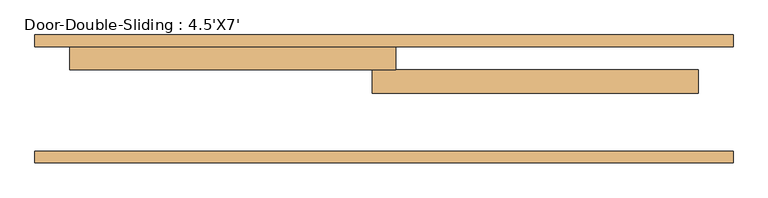
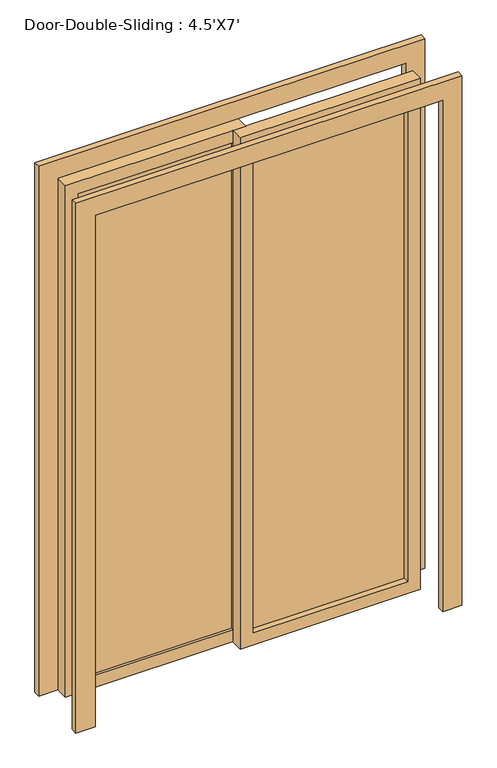
"""IFC4 building model written with IfcOpenShell, lengths in millimetres: door geometry, Door-Double-Sliding : 4.5'X7'."""

from ifc_helpers import new_model, si_unit, frame, origin, place, context, project, spatial, polyline, outline, extrude, source, transform, mapped, element, save


def door_double_sliding_4_5_x7_60868813(model_context):
    return source(origin(), model_context, "Body", "SweptSolid", [
        extrude(outline(polyline([(0.0, 762.0), (2209.8, 762.0), (2209.8, -762.0), (0.0, -762.0), (0.0, -685.8), (2133.6, -685.8), (2133.6, 685.8), (0.0, 685.8), (0.0, 762.0)])), frame((0.0, 241.3, 0.0), z_axis=(0.0, 1.0, 0.0), x_axis=(0.0, 0.0, 1.0)), (0.0, 0.0, 1.0), 25.4),
        extrude(outline(polyline([(0.0, -762.0), (0.0, -685.8), (2133.6, -685.8), (2133.6, 685.8), (0.0, 685.8), (0.0, 762.0), (2209.8, 762.0), (2209.8, -762.0), (0.0, -762.0)])), frame((0.0, -12.7, 0.0), z_axis=(0.0, 1.0, 0.0), x_axis=(0.0, 0.0, 1.0)), (0.0, 0.0, 1.0), 25.4),
        extrude(outline(polyline([(2133.6, 25.4), (2133.6, -685.8), (0.0, -685.8), (0.0, 25.4), (2133.6, 25.4)]), holes=[polyline([(2082.8, -25.4), (50.8, -25.4), (50.8, -635.0), (2082.8, -635.0), (2082.8, -25.4)])]), frame((0.0, 190.5, 0.0), z_axis=(0.0, 1.0, 0.0), x_axis=(0.0, 0.0, 1.0)), (0.0, 0.0, 1.0), 50.8),
        extrude(outline(polyline([(2133.6, -25.4), (0.0, -25.4), (0.0, 685.8), (2133.6, 685.8), (2133.6, -25.4)]), holes=[polyline([(2082.8, 25.4), (2082.8, 635.0), (50.8, 635.0), (50.8, 25.4), (2082.8, 25.4)])]), frame((0.0, 139.7, 0.0), z_axis=(0.0, 1.0, 0.0), x_axis=(0.0, 0.0, 1.0)), (0.0, 0.0, 1.0), 50.8),
        extrude(outline(polyline([(-25.4, 200.025), (-635.0, 200.025), (-635.0, 206.375), (-25.4, 206.375), (-25.4, 200.025)])), frame((0.0, 0.0, 50.8), z_axis=(0.0, 0.0, 1.0), x_axis=(1.0, 0.0, 0.0)), (0.0, 0.0, 1.0), 2032.0),
        extrude(outline(polyline([(25.4, 168.275), (635.0, 168.275), (635.0, 161.925), (25.4, 161.925), (25.4, 168.275)])), frame((0.0, 0.0, 50.8), z_axis=(0.0, 0.0, 1.0), x_axis=(1.0, 0.0, 0.0)), (0.0, 0.0, 1.0), 2032.0),
    ])


if __name__ == "__main__":
    model = new_model("IFC4")
    model_context = context("Model", 3, world=origin())
    ifc_project = project(units=[si_unit("LENGTHUNIT", "METRE", prefix="MILLI")], contexts=[model_context])
    site = spatial("IfcSite", under=ifc_project)
    building = spatial("IfcBuilding", under=site)
    placement = place(None, origin())
    door_double_sliding_4_5_x7_shape = door_double_sliding_4_5_x7_60868813(model_context)
    element("IfcDoor", 1, ObjectType="Door-Double-Sliding : 4.5'X7'", at=placement, inside=building, context=model_context, shape_type="MappedRepresentation", body=[
        mapped(door_double_sliding_4_5_x7_shape, transform((0.0, 0.0, 0.0), x_axis=(1.0, 0.0, 0.0), y_axis=(0.0, 1.0, 0.0), z_axis=(0.0, 0.0, 1.0))),
    ])
    save(model, "model.ifc")

# Revit data of these elements
# Type "Door-Double-Sliding : 4.5'X7'"
#   Type Mark = "14"
#   Construction Type Id = "opn-d45"
#   Assembly Code = "C1020"
#   Analytic Construction = "Wood frame, double glass door "
#   Thickness = 0' - 2"
#   Thermal Resistance (R) = 1.8150 (h·ft²·°F)/BTU
#   Heat Transfer Coefficient (U) = 0.5510 BTU/(h·ft²·°F)
#   Height = 7' - 0"
#   Rail Width = 0' - 2"
#   Stiles = 0' - 2"
#   Trim Projection Ext = 0' - 1"
#   Trim Projection Int = 0' - 1"
#   Trim Width = 0' - 3"
#   Width = 4' - 6"
#   Define Thermal Properties by = 1
#   Glazing = Glass
#   Panel Material = Wood - Birch - Solid Stained Light Low Gloss
#   Trim Material = Paint - Sienna
#   Visual Light Transmittance = 0
#   Solar Heat Gain Coefficient = 0
#   Function = (empty or 0)
#   Wall Closure = (empty or 0)
# Element 1 (IfcDoor, "Door-Double-Sliding : 4.5'X7'")
#   Materials on its faces: "Paint - Sienna", "Wood - Birch - Solid Stained Light Low Gloss", "Glass"
# Materials
#   "Glass": class "Glass", colour RGB 0 128 192, transparency 0.75, Description = "Soda Lime Glass", Cost = 0
#   "Wood - Birch - Solid Stained Light Low Gloss": class "Wood", colour RGB 210 159 95, transparency 0, Cost = 0
#   "Paint - Sienna": colour RGB 118 70 51, transparency 0, Cost = 0
